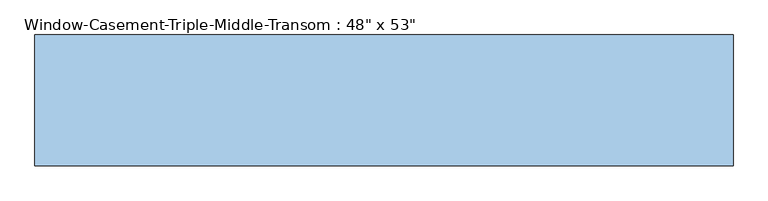
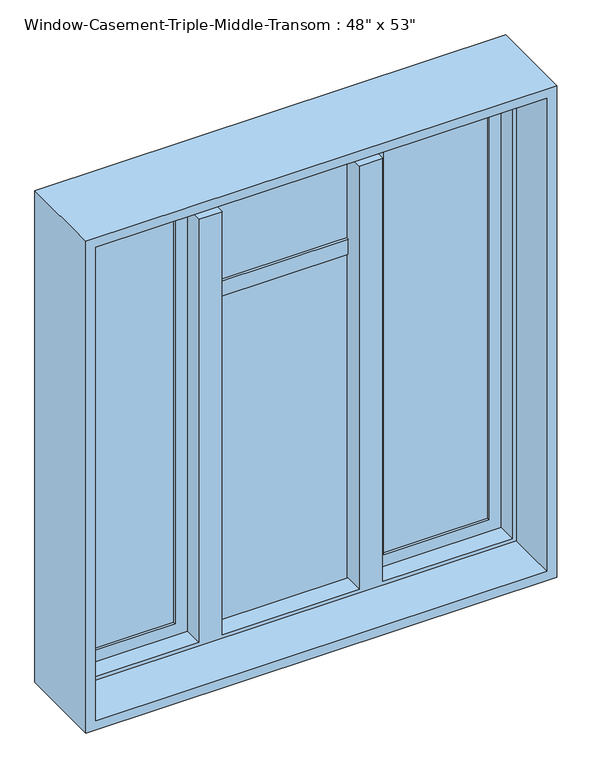
"""IFC4 building model written with IfcOpenShell, lengths in millimetres: window geometry."""

from ifc_helpers import new_model, si_unit, frame, origin, place, context, project, spatial, polyline, outline, extrude, faceted_brep, source, transform, mapped, element, save


def window_273a115f(model_context):
    return source(origin(), model_context, "Body", "SolidModel", [
        extrude(outline(polyline([(2235.2, 228.6), (939.8, 228.6), (939.8, 584.2), (2235.2, 584.2), (2235.2, 228.6)]), holes=[polyline([(2193.3296875, 542.3296875), (981.6703125, 542.3296875), (981.6703125, 270.4703125), (2193.3296875, 270.4703125), (2193.3296875, 542.3296875)])]), frame((0.0, 73.025, 0.0), z_axis=(0.0, 1.0, 0.0), x_axis=(0.0, 0.0, 1.0)), (0.0, 0.0, 1.0), 31.75),
        extrude(outline(polyline([(2235.2, -584.2), (939.8, -584.2), (939.8, -228.6), (2235.2, -228.6), (2235.2, -584.2)]), holes=[polyline([(2193.3296875, -270.4703125), (981.6703125, -270.4703125), (981.6703125, -542.3296875), (2193.3296875, -542.3296875), (2193.3296875, -270.4703125)])]), frame((0.0, 73.025, 0.0), z_axis=(0.0, 1.0, 0.0), x_axis=(0.0, 0.0, 1.0)), (0.0, 0.0, 1.0), 31.75),
        extrude(outline(polyline([(-270.4703125, 98.425), (-270.4703125, 92.075), (-542.3296875, 92.075), (-542.3296875, 98.425), (-270.4703125, 98.425)])), frame((0.0, 0.0, 949.9203125), z_axis=(0.0, 0.0, 1.0), x_axis=(1.0, 0.0, 0.0)), (0.0, 0.0, 1.0), 1275.159375),
        extrude(outline(polyline([(-270.4703125, 85.725), (-270.4703125, 79.375), (-542.3296875, 79.375), (-542.3296875, 85.725), (-270.4703125, 85.725)])), frame((0.0, 0.0, 949.9203125), z_axis=(0.0, 0.0, 1.0), x_axis=(1.0, 0.0, 0.0)), (0.0, 0.0, 1.0), 1275.159375),
        extrude(outline(polyline([(542.3296875, 98.425), (542.3296875, 92.075), (270.4703125, 92.075), (270.4703125, 98.425), (542.3296875, 98.425)])), frame((0.0, 0.0, 949.9203125), z_axis=(0.0, 0.0, 1.0), x_axis=(1.0, 0.0, 0.0)), (0.0, 0.0, 1.0), 1275.159375),
        extrude(outline(polyline([(542.3296875, 85.725), (542.3296875, 79.375), (270.4703125, 79.375), (270.4703125, 85.725), (542.3296875, 85.725)])), frame((0.0, 0.0, 949.9203125), z_axis=(0.0, 0.0, 1.0), x_axis=(1.0, 0.0, 0.0)), (0.0, 0.0, 1.0), 1275.159375),
        extrude(outline(polyline([(177.8, 104.775), (177.8, 73.025), (-177.8, 73.025), (-177.8, 104.775), (177.8, 104.775)])), frame((0.0, 0.0, 1835.8048438), z_axis=(0.0, 0.0, 1.0), x_axis=(1.0, 0.0, 0.0)), (0.0, 0.0, 1.0), 41.8703125),
        extrude(outline(polyline([(177.8, 98.425), (177.8, 92.075), (-177.8, 92.075), (-177.8, 98.425), (177.8, 98.425)])), frame((0.0, 0.0, 939.8), z_axis=(0.0, 0.0, 1.0), x_axis=(1.0, 0.0, 0.0)), (0.0, 0.0, 1.0), 896.0048437),
        extrude(outline(polyline([(177.8, 85.725), (177.8, 79.375), (-177.8, 79.375), (-177.8, 85.725), (177.8, 85.725)])), frame((0.0, 0.0, 939.8), z_axis=(0.0, 0.0, 1.0), x_axis=(1.0, 0.0, 0.0)), (0.0, 0.0, 1.0), 896.0048437),
        extrude(outline(polyline([(177.8, 98.425), (177.8, 92.075), (-177.8, 92.075), (-177.8, 98.425), (177.8, 98.425)])), frame((0.0, 0.0, 1877.6751563), z_axis=(0.0, 0.0, 1.0), x_axis=(1.0, 0.0, 0.0)), (0.0, 0.0, 1.0), 357.5248438),
        extrude(outline(polyline([(177.8, 85.725), (177.8, 79.375), (-177.8, 79.375), (-177.8, 85.725), (177.8, 85.725)])), frame((0.0, 0.0, 1877.6751563), z_axis=(0.0, 0.0, 1.0), x_axis=(1.0, 0.0, 0.0)), (0.0, 0.0, 1.0), 357.5248438),
        faceted_brep([(-584.2, 73.025, 2235.2), (-584.2, 114.3, 2235.2), (584.2, 114.3, 2235.2), (584.2, 73.025, 2235.2), (-574.0796875, 22.225, 2225.0796875), (-574.0796875, 73.025, 2225.0796875), (574.0796875, 73.025, 2225.0796875), (574.0796875, 22.225, 2225.0796875), (-584.2, -114.3, 2235.2), (-584.2, 22.225, 2235.2), (584.2, 22.225, 2235.2), (584.2, -114.3, 2235.2), (-609.6, 114.3, 2260.6), (-609.6, -114.3, 2260.6), (609.6, -114.3, 2260.6), (609.6, 114.3, 2260.6), (584.2, 114.3, 939.8), (584.2, 73.025, 939.8), (574.0796875, 73.025, 949.9203125), (574.0796875, 22.225, 949.9203125), (584.2, 22.225, 939.8), (584.2, -114.3, 939.8), (609.6, -114.3, 914.4), (609.6, 114.3, 914.4), (228.6, 73.025, 939.8), (-584.2, 114.3, 939.8), (-584.2, 73.025, 939.8), (-228.6, 73.025, 939.8), (-228.6, 111.125, 939.8), (-177.8, 111.125, 939.8), (-177.8, 73.025, 939.8), (177.8, 73.025, 939.8), (177.8, 111.125, 939.8), (228.6, 111.125, 939.8), (238.7203125, 73.025, 949.9203125), (238.7203125, 22.225, 949.9203125), (-574.0796875, 73.025, 949.9203125), (-574.0796875, 22.225, 949.9203125), (-238.7203125, 22.225, 949.9203125), (-238.7203125, 73.025, 949.9203125), (177.8, 73.025, 949.9203125), (-177.8, 73.025, 949.9203125), (-177.8, 22.225, 949.9203125), (177.8, 22.225, 949.9203125), (-584.2, 22.225, 939.8), (-584.2, -114.3, 939.8), (-609.6, -114.3, 914.4), (-609.6, 114.3, 914.4), (228.6, 73.025, 2108.2), (238.7203125, 73.025, 2108.2), (-238.7203125, 73.025, 2108.2), (-228.6, 73.025, 2108.2), (-177.8, 111.125, 2108.2), (-228.6, 111.125, 2108.2), (-238.7203125, 22.225, 2108.2), (-177.8, 22.225, 2108.2), (228.6, 111.125, 2108.2), (177.8, 111.125, 2108.2), (177.8, 22.225, 2108.2), (238.7203125, 22.225, 2108.2)], [[[0, 1, 2, 3]], [[4, 5, 6, 7]], [[8, 9, 10, 11]], [[12, 13, 14, 15]], [[3, 2, 16, 17]], [[7, 6, 18, 19]], [[11, 10, 20, 21]], [[15, 14, 22, 23]], [[24, 17, 16, 25, 26, 27, 28, 29, 30, 31, 32, 33]], [[19, 18, 34, 35]], [[36, 37, 38, 39]], [[40, 41, 42, 43]], [[21, 20, 44, 45]], [[23, 22, 46, 47]], [[1, 0, 26, 25]], [[0, 3, 17, 24, 48, 49, 34, 18, 6, 5, 36, 39, 50, 51, 27, 26]], [[41, 40, 31, 30]], [[5, 4, 37, 36]], [[9, 8, 45, 44]], [[14, 13, 46, 22], [8, 11, 21, 45]], [[13, 12, 47, 46]], [[12, 15, 23, 47], [2, 1, 25, 16]], [[52, 53, 51, 50, 54, 55]], [[56, 57, 58, 59, 49, 48]], [[53, 52, 29, 28]], [[27, 51, 53, 28]], [[52, 55, 42, 41, 30, 29]], [[57, 56, 33, 32]], [[58, 57, 32, 31, 40, 43]], [[56, 48, 24, 33]], [[54, 50, 39, 38]], [[49, 59, 35, 34]], [[10, 9, 44, 20], [4, 7, 19, 35, 59, 58, 43, 42, 55, 54, 38, 37]]]),
    ])


if __name__ == "__main__":
    model = new_model("IFC4")
    model_context = context("Model", 3, world=origin())
    ifc_project = project(units=[si_unit("LENGTHUNIT", "METRE", prefix="MILLI")], contexts=[model_context])
    site = spatial("IfcSite", under=ifc_project)
    building = spatial("IfcBuilding", under=site)
    placement = place(None, origin())
    window_shape = window_273a115f(model_context)
    element("IfcWindow", 1, ObjectType="Window-Casement-Triple-Middle-Transom : 48\" x 53\"", at=placement, inside=building, context=model_context, shape_type="MappedRepresentation", body=[
        mapped(window_shape, transform((0.0, 0.0, 0.0), x_axis=(1.0, 0.0, 0.0), y_axis=(0.0, 1.0, 0.0), z_axis=(0.0, 0.0, 1.0))),
    ])
    save(model, "model.ifc")

# Revit data of these elements
# Type "Window-Casement-Triple-Middle-Transom : 48\" x 53\""
#   Type Mark = "18"
#   Fire Rating = "0.5h"
#   Assembly Code = "B2020100"
#   Analytic Construction = "Double glazing - domestic"
#   Window Width = 1' - 4"
#   Window Inset [instance default] = 0' - 0 5/8"
#   Wall Thickness [instance default] = 0' - 6"
#   Visual Light Transmittance = 0.81
#   Transom Height Ratio = 0.3
#   Thermal Resistance (R) = 1.8146 (h·ft²·°F)/BTU
#   Solar Heat Gain Coefficient = 0.76
#   Rough Width = 4' - 0 1/2"
#   Rough Height = 4' - 5 1/2"
#   Heat Transfer Coefficient (U) = 0.5511 BTU/(h·ft²·°F)
#   Height = 4' - 5"
#   Transom Height = 1' - 3.9"
#   Frame Gap 3 [instance default] = 0' - 1 83/128"
#   Frame Gap 2 [instance default] = 0' - 0 5/8"
#   Frame Gap 1 = 0' - 1 51/128"
#   Default Sill Height = 3' - 0"
#   Width = 4' - 0"
#   Frame Material = Metal - Aluminum
#   Glass Panel Material = Glass
#   Wall Closure = (empty or 0)
# Element 1 (IfcWindow, "Window-Casement-Triple-Middle-Transom : 48\" x 53\"")
#   Wall Thickness = 0' - 9"
#   Materials on its faces: "Metal - Aluminum", "Glass"
# Materials
#   "Metal - Aluminum": class "Metal", colour RGB 247 247 247, transparency 0
#   "Glass": class "Glass", colour RGB 0 128 192, transparency 0.75, Description = "Soda Lime Glass", Cost = 0
